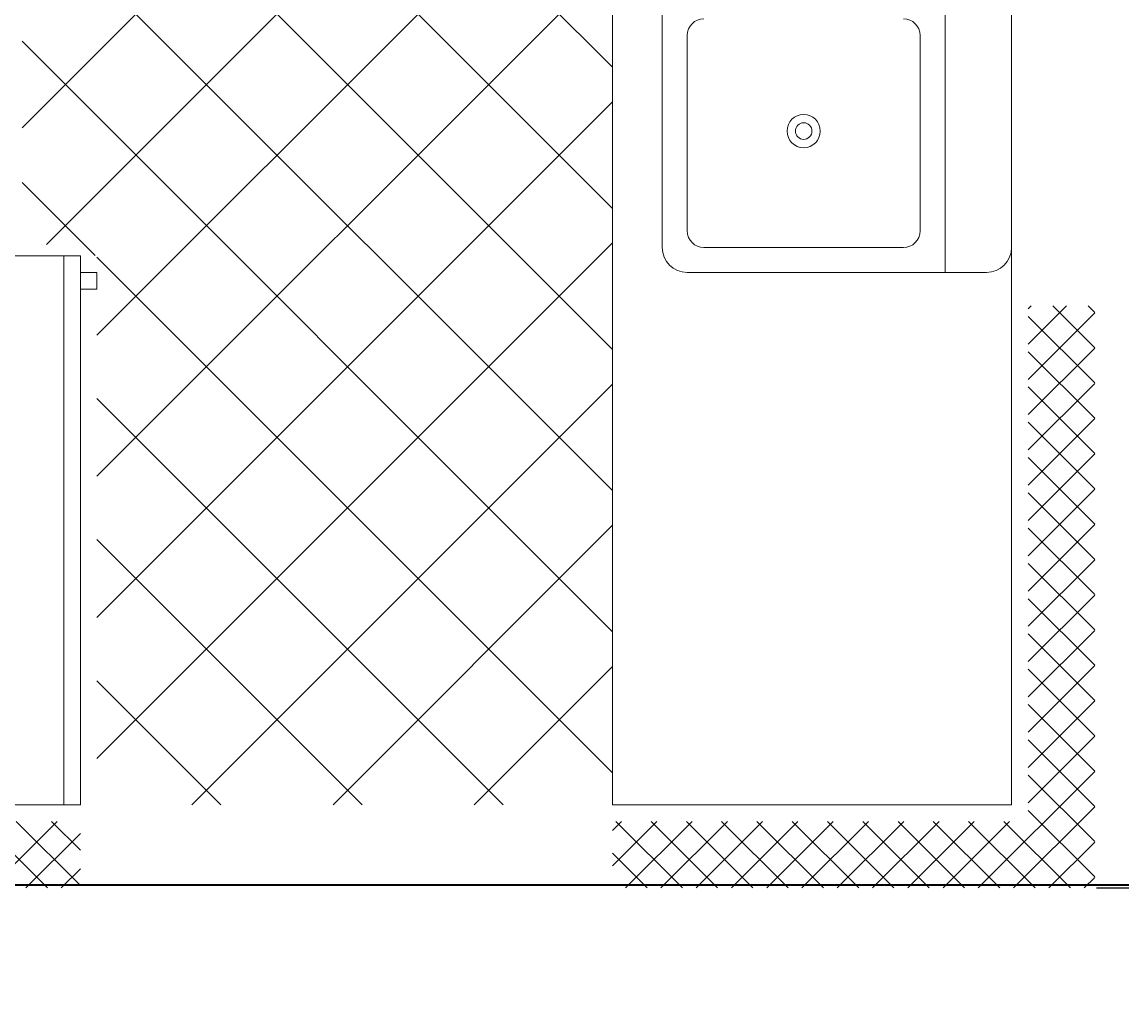
# Model space of a CAD drawing. Units: inches. Extents: x 4159 to 4826, y 299 to 1026.
# Tile 14 of 37: x 4218 to 4255, y 596 to 630. Entities that reach past the tile are written whole.
import ezdxf

# ---------------------------------------------------------------- set-up
doc = ezdxf.new("R2010")
doc.units = ezdxf.units.IN
for name, color, linetype, lineweight in [('A-ANNO-DIMS', 2, 'Continuous', 18), ('A-FLOR-FIXT', 9, 'Continuous', 18), ('A-WALL', 7, 'Continuous', 35)]:
    doc.layers.add(name, color=color, linetype=linetype, lineweight=lineweight)
doc.styles.get("Standard").update_dxf_attribs({"font": 'arial.ttf'})
doc.dimstyles.get("Standard").update_dxf_attribs({"dimtxt": 0.18, "dimasz": 0.18, "dimexe": 0.18, "dimexo": 0.0625, "dimgap": 0.09, "dimtad": 0, "dimtih": 1, "dimtoh": 1, "dimdec": 4, "dimzin": 0, "dimdsep": 46, "dimtxsty": 'Standard', "dimcen": 0.09, "dimadec": 0, "dimazin": 0, "dimtfac": 1, "dimtdec": 4, "dimtofl": 0, "dimtmove": 0, "dimatfit": 3, "dimfxl": 1, "dimtolj": 1, "dimtzin": 0, "dimarcsym": 0})

# ---------------------------------------------------------------- blocks, each defined once
blk = doc.blocks.new('Kitchen Layout - 7 x 8 ft')
for p, q in [((-5, 57.981), (-1, 61.981)), ((-1, 57.394), (-5, 61.394)), ((-4.86, 56), (-1, 59.86)), ((-1.727, 56), (-5, 59.273)), ((10.397, 24), (45.897, 59.5)), ((18.882, 24), (54.382, 59.5)), ((27.368, 24), (62.868, 59.5)), ((33.025, 55.114), (37.412, 59.5)), ((35.853, 24), (71.353, 59.5)), ((76.199, 24), (40.699, 59.5)), ((-2.739, 56), (-1, 57.739)), ((67.714, 24), (33.675, 58.038)), ((-3.848, 56), (-5, 57.152)), ((0, 57), (33, 57)), ((44.338, 24), (77.838, 57.5)), ((31, 55), (31, 56)), ((32, 56), (32, 55)), ((0, 30.574), (24.426, 55)), ((0, 39.059), (15.941, 55)), ((0, 47.544), (7.456, 55)), ((1.912, 24), (32.912, 55)), ((33.772, 24), (2.773, 55)), ((42.258, 24), (11.258, 55)), ((50.743, 24), (19.743, 55)), ((59.228, 24), (28.228, 55)), ((32, 55), (31, 55)), ((25.287, 24), (0, 49.287)), ((16.802, 24), (0, 40.802)), ((8.317, 24), (0, 32.317)), ((-5, 21.919), (-2.919, 24)), ((-1, 21.332), (-3.668, 24)), ((-1, 23.453), (-1.547, 24)), ((0, 24), (96, 24)), ((0, 0), (0, 24)), ((-5, 19.797), (-1, 23.797)), ((-1, 19.21), (-5, 23.21)), ((-5, 17.676), (-1, 21.676)), ((-1, 17.089), (-5, 21.089)), ((-5, 15.555), (-1, 19.555)), ((-1, 14.968), (-5, 18.968)), ((-5, 13.433), (-1, 17.433)), ((-1, 12.847), (-5, 16.847)), ((-5, 11.312), (-1, 15.312)), ((-1, 10.725), (-5, 14.725)), ((-5, 9.191), (-1, 13.191)), ((-1, 8.604), (-5, 12.604)), ((-5, 7.069), (-1, 11.069)), ((-1, 6.483), (-5, 10.483)), ((-5, 4.948), (-1, 8.948)), ((-1, 4.361), (-5, 8.361)), ((-5, 2.827), (-1, 6.827)), ((-1, 2.24), (-5, 6.24)), ((-5, 0.705), (-1, 4.705)), ((-1, 0.119), (-5, 4.119)), ((64, 4), (32, 4)), ((-5, -1.416), (-1, 2.584)), ((1.997, -5), (-5, 1.997)), ((-5, -3.537), (-1, 0.463)), ((96, 0), (0, 0)), ((-0.124, -5), (-5, -0.124)), ((-4.342, -5), (-0.342, -1)), ((-2.22, -5), (1.78, -1)), ((-0.099, -5), (3.901, -1)), ((4.119, -5), (0.119, -1)), ((2.022, -5), (6.022, -1)), ((6.24, -5), (2.24, -1)), ((4.144, -5), (8.144, -1)), ((8.361, -5), (4.361, -1)), ((6.265, -5), (10.265, -1)), ((10.483, -5), (6.483, -1)), ((8.386, -5), (12.386, -1)), ((12.604, -5), (8.604, -1)), ((10.508, -5), (14.508, -1)), ((14.725, -5), (10.725, -1)), ((12.629, -5), (16.629, -1)), ((16.847, -5), (12.847, -1)), ((14.75, -5), (18.75, -1)), ((18.968, -5), (14.968, -1)), ((16.872, -5), (20.872, -1)), ((21.089, -5), (17.089, -1)), ((18.993, -5), (22.993, -1)), ((23.21, -5), (19.21, -1)), ((21.114, -5), (25.114, -1)), ((25.332, -5), (21.332, -1)), ((23.236, -5), (27.236, -1)), ((27.453, -5), (23.453, -1)), ((25.357, -5), (29.357, -1)), ((29.574, -5), (25.574, -1)), ((30, -3.304), (27.696, -1)), ((30, -1.183), (29.817, -1)), ((-2.245, -5), (-5, -2.245)), ((27.478, -5), (30, -2.478)), ((-4.367, -5), (-5, -4.367)), ((29.6, -5), (30, -4.6))]:
    blk.add_line(p, q)
blk.add_lwpolyline([(0, 56), (0, 84), (33, 84), (33, 56)], close=True)
for points in [[(33.5, 21), (62.5, 21)], [(32, 1.5), (32, 19.5)], [(34.5, 19.5), (46.25, 19.5)], [(33.5, 6.5), (33.5, 18.5)], [(46.25, 5.5), (34.5, 5.5)], [(62.5, 0), (33.5, 0)]]:
    blk.add_lwpolyline(points)
for radius in [1, 0.5]:
    blk.add_circle((40.5, 12.5), radius)
for centre, radius, start, end in [((33.5, 19.5), 1.5, 90, 180), ((34.5, 18.5), 1, 90, 180), ((46.25, 18.5), 1, 0, 90), ((34.5, 6.5), 1, 180, 270), ((46.25, 6.5), 1, 270, 0), ((33.5, 1.5), 1.5, 180, 270)]:
    blk.add_arc(centre, radius, start, end)
blk = doc.blocks.new('*D39')
at = {"layer": 'A-ANNO-DIMS', "color": 0, "lineweight": -2, "transparency": 16777216}
for p, q in [((4254.612, 660.06), (4263.714, 660.06)), ((4263.534, 659.88), (4263.534, 630.296)), ((4263.534, 600.346), (4263.534, 629.93)), ((4254.612, 600.166), (4263.714, 600.166))]:
    blk.add_line(p, q, dxfattribs=at)
at = {"layer": 'A-ANNO-DIMS', "color": 0, "transparency": 16777216}
for points in [[(4263.504, 659.88), (4263.564, 659.88), (4263.534, 660.06)], [(4263.504, 600.346), (4263.564, 600.346), (4263.534, 600.166)]]:
    blk.add_solid(points, dxfattribs=at)
at = {"layer": 'Defpoints', "color": 0, "transparency": 16777216}
for p in [(4254.55, 660.06), (4263.534, 660.06), (4254.55, 600.166)]:
    blk.add_point(p, dxfattribs=at)
at = {"layer": 'A-ANNO-DIMS', "color": 0, "transparency": 16777216, "insert": (4263.534, 630.113), "char_height": 0.18, "attachment_point": 5}
blk.add_mtext('\\A1;KITCHEN 60 TYP.', dxfattribs=at)
blk = doc.blocks.new('*D44')
at = {"layer": 'A-ANNO-DIMS', "color": 0, "lineweight": -2, "transparency": 16777216}
for p, q in [((4287.263, 963.093), (4158.88, 963.093)), ((4159.06, 962.913), (4159.06, 647.826)), ((4159.06, 332.375), (4159.06, 647.462)), ((4447.248, 332.195), (4158.88, 332.195))]:
    blk.add_line(p, q, dxfattribs=at)
at = {"layer": 'A-ANNO-DIMS', "color": 0, "transparency": 16777216}
for points in [[(4159.03, 962.913), (4159.09, 962.913), (4159.06, 963.093)], [(4159.03, 332.375), (4159.09, 332.375), (4159.06, 332.195)]]:
    blk.add_solid(points, dxfattribs=at)
at = {"layer": 'Defpoints', "color": 0, "transparency": 16777216}
for p in [(4287.326, 963.093), (4159.06, 332.195), (4447.31, 332.195)]:
    blk.add_point(p, dxfattribs=at)
at = {"layer": 'A-ANNO-DIMS', "color": 0, "transparency": 16777216, "insert": (4159.06, 647.644), "char_height": 0.18, "attachment_point": 5}
blk.add_mtext('\\A1;630.9', dxfattribs=at)

msp = doc.modelspace()

# ---------------------------------------------------------------- linework, layer by layer
at = {"layer": 'A-WALL'}
msp.add_line((4277.31, 600.254), (4201.31, 600.254), dxfattribs=at)

# ---------------------------------------------------------------- block references
at = {"layer": 'A-FLOR-FIXT', "xscale": 0.5650329326971529, "yscale": 0.5650329326971529, "zscale": 0.5650329326971529, "rotation": 90}
msp.add_blockref('Kitchen Layout - 7 x 8 ft', (4251.725, 602.991), dxfattribs=at)

# ---------------------------------------------------------------- dimensions: what is measured, and where the dimension line sits
at = {"layer": 'A-ANNO-DIMS'}
dim = msp.add_linear_dim(base=(4159.06, 332.195), p1=(4287.326, 963.093), p2=(4447.31, 332.195), angle=90, dimstyle='Standard', override={"dimdec": 1, "dimlfac": 1, "dimrnd": 0, "dimzin": 0, "dimdsep": 46, "dimlunit": 2}, dxfattribs=at)
dim.commit()
dim.dimension.update_dxf_attribs({"geometry": '*D44', "text_midpoint": (4159.06, 647.644)})
dim = msp.add_linear_dim(base=(4263.534, 660.06), p1=(4254.55, 600.166), p2=(4254.55, 660.06), angle=90, text='KITCHEN <> TYP.', dimstyle='Standard', override={"dimdec": 0, "dimlfac": 1, "dimrnd": 0, "dimzin": 0, "dimdsep": 46, "dimlunit": 2}, dxfattribs=at)
dim.commit()
dim.dimension.update_dxf_attribs({"geometry": '*D39', "text_midpoint": (4263.534, 630.113)})

doc.saveas('drawing.dxf')
